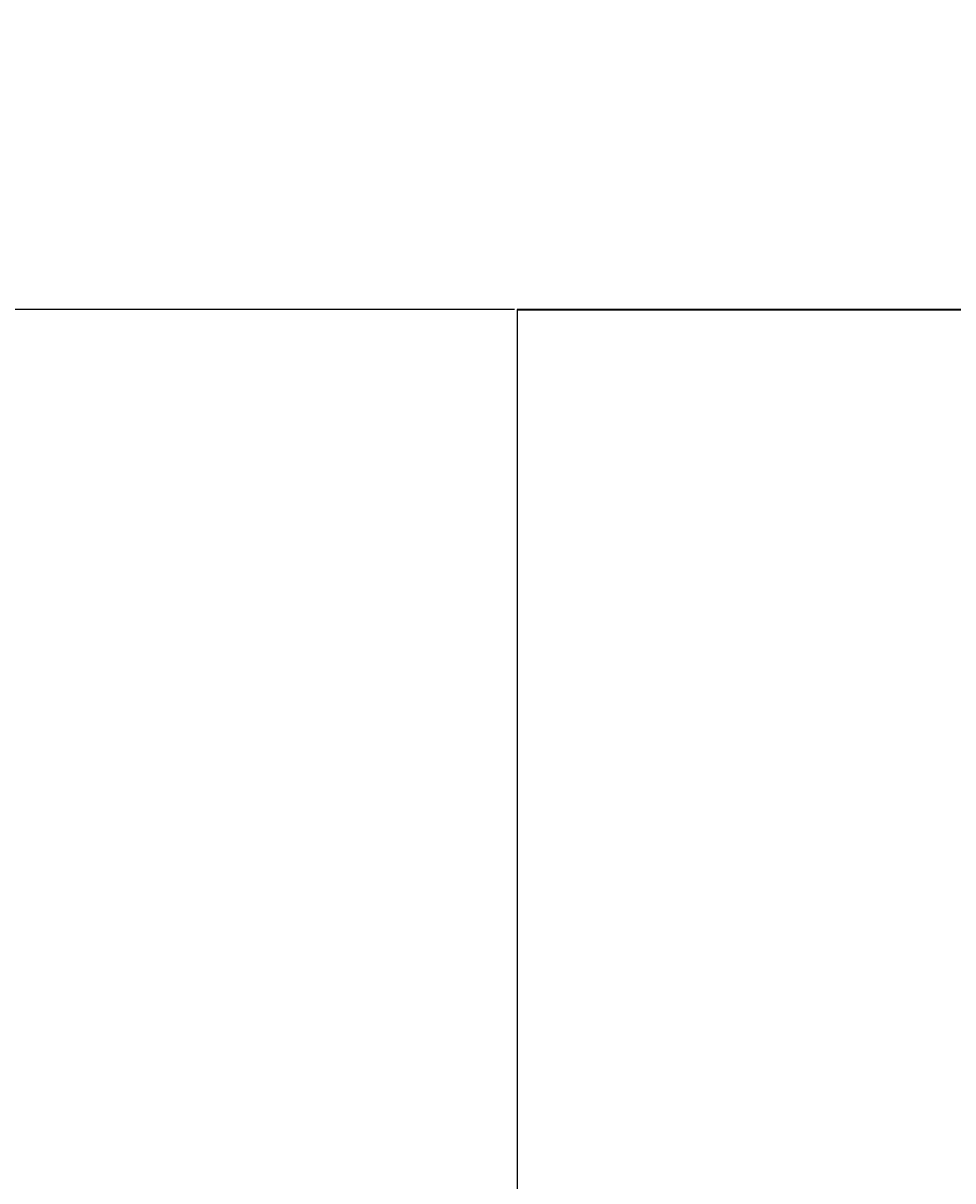
# Model space of a CAD drawing. Units: inches. Extents: x 1885 to 2748, y 783 to 2421.
# Tile 32 of 117: x 1969 to 1991, y 1503 to 1531. Entities that reach past the tile are written whole.
import ezdxf

# ---------------------------------------------------------------- set-up
doc = ezdxf.new("R2010")
doc.units = ezdxf.units.IN
for name, color, linetype, lineweight in [('A-ANNO-DIMS', 2, 'Continuous', 18), ('A-FLOR-BALC', 7, 'Continuous', 25), ('A-WALL', 7, 'Continuous', 35)]:
    doc.layers.add(name, color=color, linetype=linetype, lineweight=lineweight)
doc.styles.get("Standard").update_dxf_attribs({"font": 'arial.ttf'})
doc.dimstyles.get("Standard").update_dxf_attribs({"dimtxt": 0.18, "dimasz": 0.18, "dimexe": 0.18, "dimexo": 0.0625, "dimgap": 0.09, "dimtad": 0, "dimtih": 1, "dimtoh": 1, "dimdec": 4, "dimzin": 0, "dimdsep": 46, "dimtxsty": 'Standard', "dimcen": 0.09, "dimadec": 0, "dimazin": 0, "dimtfac": 1, "dimtdec": 4, "dimtofl": 0, "dimtmove": 0, "dimatfit": 3, "dimfxl": 1, "dimtolj": 1, "dimtzin": 0, "dimarcsym": 0})

# ---------------------------------------------------------------- blocks, each defined once
blk = doc.blocks.new('*D45')
at = {"layer": 'A-ANNO-DIMS', "color": 0, "lineweight": -2, "transparency": 16777216}
for p, q in [((1980.711, 1524.006), (1902.844, 1524.006)), ((1903.024, 1523.826), (1903.024, 1290.937)), ((1903.024, 1057.686), (1903.024, 1290.574)), ((1971.211, 1057.506), (1902.844, 1057.506))]:
    blk.add_line(p, q, dxfattribs=at)
at = {"layer": 'A-ANNO-DIMS', "color": 0, "transparency": 16777216}
for points in [[(1902.994, 1523.826), (1903.054, 1523.826), (1903.024, 1524.006)], [(1902.994, 1057.686), (1903.054, 1057.686), (1903.024, 1057.506)]]:
    blk.add_solid(points, dxfattribs=at)
at = {"layer": 'Defpoints', "color": 0, "transparency": 16777216}
for p in [(1903.024, 1524.006), (1980.774, 1524.006), (1971.274, 1057.506)]:
    blk.add_point(p, dxfattribs=at)
at = {"layer": 'A-ANNO-DIMS', "color": 0, "transparency": 16777216, "insert": (1903.024, 1290.756), "char_height": 0.18, "attachment_point": 5}
blk.add_mtext('\\A1;466.5', dxfattribs=at)
blk = doc.blocks.new('*D46')
at = {"layer": 'A-ANNO-DIMS', "color": 0, "lineweight": -2, "transparency": 16777216}
for p, q in [((1980.711, 1558.006), (1902.844, 1558.006)), ((1903.024, 1557.826), (1903.024, 1541.188)), ((1903.024, 1524.186), (1903.024, 1540.824)), ((1980.711, 1524.006), (1902.844, 1524.006))]:
    blk.add_line(p, q, dxfattribs=at)
at = {"layer": 'A-ANNO-DIMS', "color": 0, "transparency": 16777216}
for points in [[(1902.994, 1557.826), (1903.054, 1557.826), (1903.024, 1558.006)], [(1902.994, 1524.186), (1903.054, 1524.186), (1903.024, 1524.006)]]:
    blk.add_solid(points, dxfattribs=at)
at = {"layer": 'Defpoints', "color": 0, "transparency": 16777216}
for p in [(1903.024, 1558.006), (1980.774, 1558.006), (1980.774, 1524.006)]:
    blk.add_point(p, dxfattribs=at)
at = {"layer": 'A-ANNO-DIMS', "color": 0, "transparency": 16777216, "insert": (1903.024, 1541.006), "char_height": 0.18, "attachment_point": 5}
blk.add_mtext('\\A1;34', dxfattribs=at)

msp = doc.modelspace()

# ---------------------------------------------------------------- linework, layer by layer
at = {"layer": 'A-FLOR-BALC'}
msp.add_line((1980.774, 1524.006), (1980.774, 1383.006), dxfattribs=at)
at = {"layer": 'A-WALL'}
msp.add_line((1980.774, 1524.006), (2044.674, 1524.006), dxfattribs=at)

# ---------------------------------------------------------------- dimensions: what is measured, and where the dimension line sits
at = {"layer": 'A-ANNO-DIMS'}
for base, p1, p2, override, picture, middle in [((1903.024, 1558.006), (1980.774, 1524.006), (1980.774, 1558.006), {"dimdec": 0, "dimlfac": 1, "dimrnd": 0, "dimzin": 0, "dimdsep": 46, "dimlunit": 2}, '*D46', (1903.024, 1541.006)), ((1903.024, 1524.006), (1971.274, 1057.506), (1980.774, 1524.006), {"dimdec": 1, "dimlfac": 1, "dimrnd": 0, "dimzin": 0, "dimdsep": 46, "dimlunit": 2}, '*D45', (1903.024, 1290.756))]:
    dim = msp.add_linear_dim(base=base, p1=p1, p2=p2, angle=90, dimstyle='Standard', override=override, dxfattribs=at)
    dim.commit()
    dim.dimension.update_dxf_attribs({"geometry": picture, "text_midpoint": middle})

doc.saveas('drawing.dxf')
